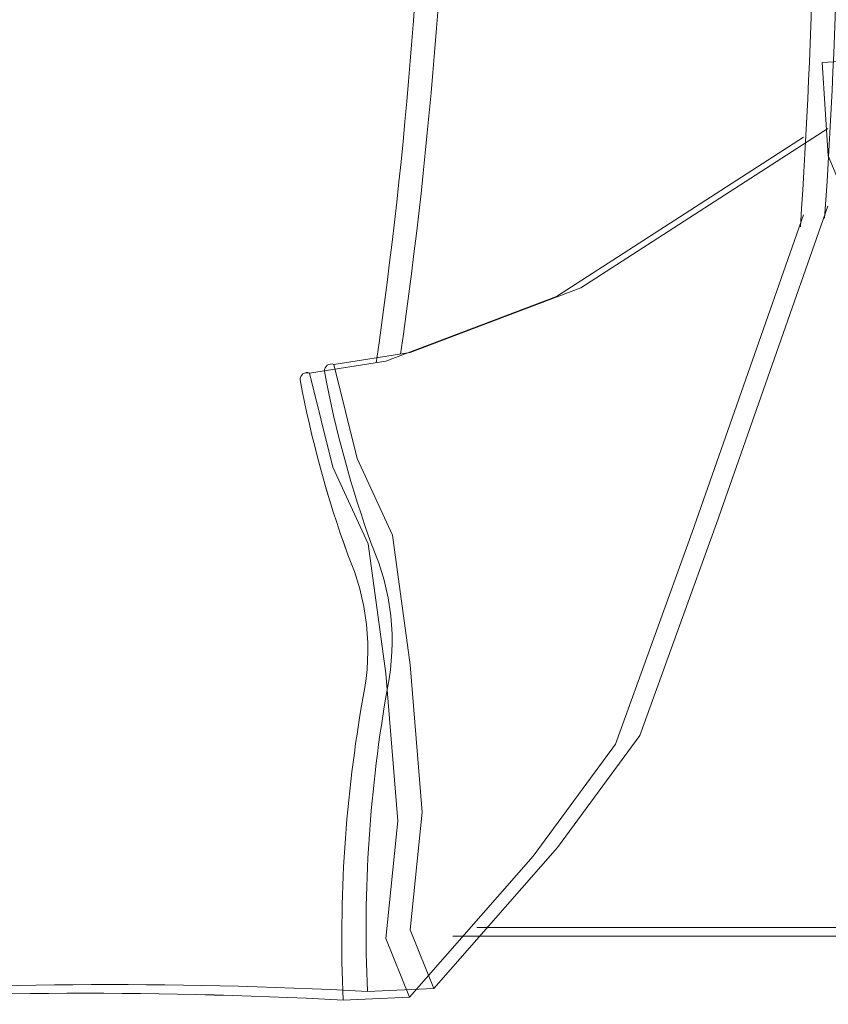
# Model space of a CAD drawing. Units: inches. Extents: x 1962 to 2771, y 1245 to 2660.
# Tile 74 of 114: x 2625.6 to 2642.5, y 2030.14 to 2050.72. Entities that reach past the tile are written whole.
import ezdxf

# ---------------------------------------------------------------- set-up
doc = ezdxf.new("R2010")
doc.units = ezdxf.units.IN
doc.layers.add('A-ANNO-DIMS', color=2, linetype='Continuous', lineweight=18)
doc.layers.add('A-FURN', color=8, linetype='Continuous', lineweight=13)
doc.styles.get("Standard").update_dxf_attribs({"font": 'arial.ttf'})
doc.dimstyles.get("Standard").update_dxf_attribs({"dimtxt": 0.18, "dimasz": 0.18, "dimexe": 0.18, "dimexo": 0.0625, "dimgap": 0.09, "dimtad": 0, "dimtih": 1, "dimtoh": 1, "dimdec": 4, "dimzin": 0, "dimdsep": 46, "dimtxsty": 'Standard', "dimcen": 0.09, "dimadec": 0, "dimazin": 0, "dimtfac": 1, "dimtdec": 4, "dimtofl": 0, "dimtmove": 0, "dimatfit": 3, "dimfxl": 1, "dimtolj": 1, "dimtzin": 0, "dimarcsym": 0})

# ---------------------------------------------------------------- blocks, each defined once
blk = doc.blocks.new('BED-PLAN')
for p, q in [((22.563, 42.207), (19.979, 39.261)), ((22.563, 42.206), (19.979, 39.261)), ((23.95, 42.27), (22.563, 42.207, 3.077)), ((23.95, 42.27), (22.563, 42.206, 3.077)), ((23.055, 40.985), (22.563, 42.207)), ((23.055, 40.985), (22.563, 42.206)), ((22.055, 42.025), (19.471, 39.08)), ((22.055, 42.025), (19.471, 39.08)), ((23.442, 42.088), (22.055, 42.025, 3.077)), ((23.442, 42.088), (22.055, 42.025, 3.077)), ((22.547, 40.803), (22.055, 42.025)), ((22.547, 40.803), (22.055, 42.025)), ((22.809, 38.523), (23.055, 40.985)), ((22.809, 38.522), (23.055, 40.985)), ((0, 40.752), (21.152, 40.752)), ((0, 40.751), (21.152, 40.751)), ((0.508, 40.933), (21.66, 40.933)), ((0.508, 40.933), (21.66, 40.933)), ((22.301, 38.341), (22.547, 40.803)), ((22.301, 38.341), (22.547, 40.803)), ((19.979, 39.261), (18.257, 36.922)), ((19.979, 39.261), (18.257, 36.922)), ((19.471, 39.08), (17.749, 36.741)), ((19.471, 39.08), (17.749, 36.741)), ((23.055, 35.445), (22.809, 38.523)), ((23.055, 35.445), (22.809, 38.522)), ((22.547, 35.263), (22.301, 38.341)), ((22.547, 35.263), (22.301, 38.341)), ((18.257, 36.922), (16.658, 32.49)), ((18.257, 36.922), (16.658, 32.49)), ((17.749, 36.741), (16.149, 32.309)), ((17.749, 36.741), (16.149, 32.309)), ((23.424, 32.737), (23.055, 35.445)), ((23.424, 32.736), (23.055, 35.445)), ((22.916, 32.555), (22.547, 35.263)), ((22.916, 32.555), (22.547, 35.263)), ((24.162, 31.136), (23.424, 32.737)), ((24.162, 31.136), (23.424, 32.736)), ((23.654, 30.955), (22.916, 32.555)), ((23.654, 30.955), (22.916, 32.555)), ((16.149, 32.309), (13.818, 25.681)), ((16.149, 32.309), (13.818, 25.681)), ((16.658, 32.49), (14.326, 25.863)), ((16.658, 32.49), (14.326, 25.862)), ((24.655, 29.167), (24.162, 31.136)), ((24.655, 29.166), (24.162, 31.136)), ((24.146, 28.985), (23.654, 30.955)), ((24.146, 28.985), (23.654, 30.955)), ((23.055, 28.92), (24.655, 29.167)), ((23.055, 28.92), (24.655, 29.166)), ((19.487, 27.566), (23.055, 28.92)), ((19.487, 27.566), (23.055, 28.92)), ((22.547, 28.739), (24.146, 28.985)), ((22.547, 28.739), (24.146, 28.985)), ((18.979, 27.385), (22.547, 28.739)), ((18.979, 27.384), (22.547, 28.739)), ((13.818, 24.054), (18.979, 27.385)), ((13.818, 24.054), (18.979, 27.384)), ((14.326, 24.236), (19.487, 27.566)), ((14.326, 24.235), (19.487, 27.566)), ((13.814, 24.626), (12.793, 27.067)), ((13.814, 24.626), (12.793, 27.066)), ((13.936, 22.676), (13.814, 24.626)), ((13.936, 22.676), (13.814, 24.626)), ((11.809, 22.543), (13.936, 22.676)), ((11.809, 22.543), (13.936, 22.676))]:
    blk.add_line(p, q)
for centre, radius, start, end in [((-4.783, 40.982), 28.761, 349.8763, 2.5657), ((-4.783, 40.982), 28.761, 349.8763, 2.5657), ((29.375, 145.064), 102.937, 266.97912, 273.83645), ((29.375, 145.063), 102.937, 266.97912, 273.83645), ((-5.291, 40.801), 28.761, 349.8763, 2.5657), ((-5.291, 40.801), 28.761, 349.8763, 2.5657), ((28.866, 144.882), 102.937, 266.97912, 273.83645), ((28.866, 144.882), 102.937, 266.97912, 273.83645), ((28.382, 34.954), 4.948, 168.6608, 203.7384), ((28.382, 34.954), 4.948, 168.6608, 203.7384), ((27.874, 34.772), 4.948, 168.6608, 203.7384), ((27.874, 34.772), 4.948, 168.6608, 203.7384), ((1.686, 24.947), 23.571, 10.6617, 19.8806), ((1.686, 24.946), 23.571, 10.6617, 19.8806), ((1.178, 24.765), 23.571, 10.6617, 19.8806), ((1.178, 24.765), 23.571, 10.6617, 19.8806), ((24.704, 29.305), 0.147, 250.2464, 1.1377), ((24.704, 29.304), 0.147, 250.2464, 1.1377), ((24.196, 29.123), 0.147, 250.2464, 1.1377), ((24.196, 29.123), 0.147, 250.2464, 1.1377), ((124.762, 14.297), 102.556, 171.78449, 186.90062), ((124.762, 14.296), 102.556, 171.78449, 186.90062), ((124.254, 14.115), 102.556, 171.78449, 186.90062), ((124.254, 14.115), 102.556, 171.78449, 186.90062), ((144.711, 16.979), 131.131, 176.08655, 186.78213), ((144.711, 16.979), 131.131, 176.08655, 186.78213), ((145.219, 17.161), 131.131, 176.08655, 186.78213), ((145.219, 17.161), 131.131, 176.08655, 186.78213)]:
    blk.add_arc(centre, radius, start, end)
blk = doc.blocks.new('*D40')
at = {"layer": 'A-ANNO-DIMS', "color": 0, "lineweight": -2, "transparency": 16777216}
for p, q in [((2072.02, 2033.906), (2072.02, 2583.474)), ((2660.807, 2524.406), (2660.807, 2583.474)), ((2072.2, 2583.294), (2366.02, 2583.294)), ((2660.627, 2583.294), (2366.808, 2583.294))]:
    blk.add_line(p, q, dxfattribs=at)
at = {"layer": 'A-ANNO-DIMS', "color": 0, "transparency": 16777216}
for points in [[(2072.2, 2583.324), (2072.2, 2583.264), (2072.02, 2583.294)], [(2660.627, 2583.324), (2660.627, 2583.264), (2660.807, 2583.294)]]:
    blk.add_solid(points, dxfattribs=at)
at = {"layer": 'Defpoints', "color": 0, "transparency": 16777216}
for p in [(2660.807, 2583.294), (2660.807, 2524.344), (2072.02, 2033.844)]:
    blk.add_point(p, dxfattribs=at)
at = {"layer": 'A-ANNO-DIMS', "color": 0, "transparency": 16777216, "insert": (2366.414, 2583.294), "char_height": 0.18, "attachment_point": 5}
blk.add_mtext('\\A1;588.8', dxfattribs=at)

msp = doc.modelspace()

# ---------------------------------------------------------------- block references
at = {"layer": 'A-FURN', "rotation": 180}
msp.add_blockref('BED-PLAN', (2656.3074, 2072.498), dxfattribs=at)

# ---------------------------------------------------------------- dimensions: what is measured, and where the dimension line sits
at = {"layer": 'A-ANNO-DIMS'}
dim = msp.add_linear_dim(base=(2660.8074, 2583.2937), p1=(2072.0204, 2033.8437), p2=(2660.8074, 2524.3437), dimstyle='Standard', override={"dimdec": 1, "dimlfac": 1, "dimrnd": 0, "dimzin": 0, "dimdsep": 46, "dimlunit": 2}, dxfattribs=at)
dim.commit()
dim.dimension.update_dxf_attribs({"geometry": '*D40', "text_midpoint": (2366.4139, 2583.2937)})

doc.saveas('drawing.dxf')
